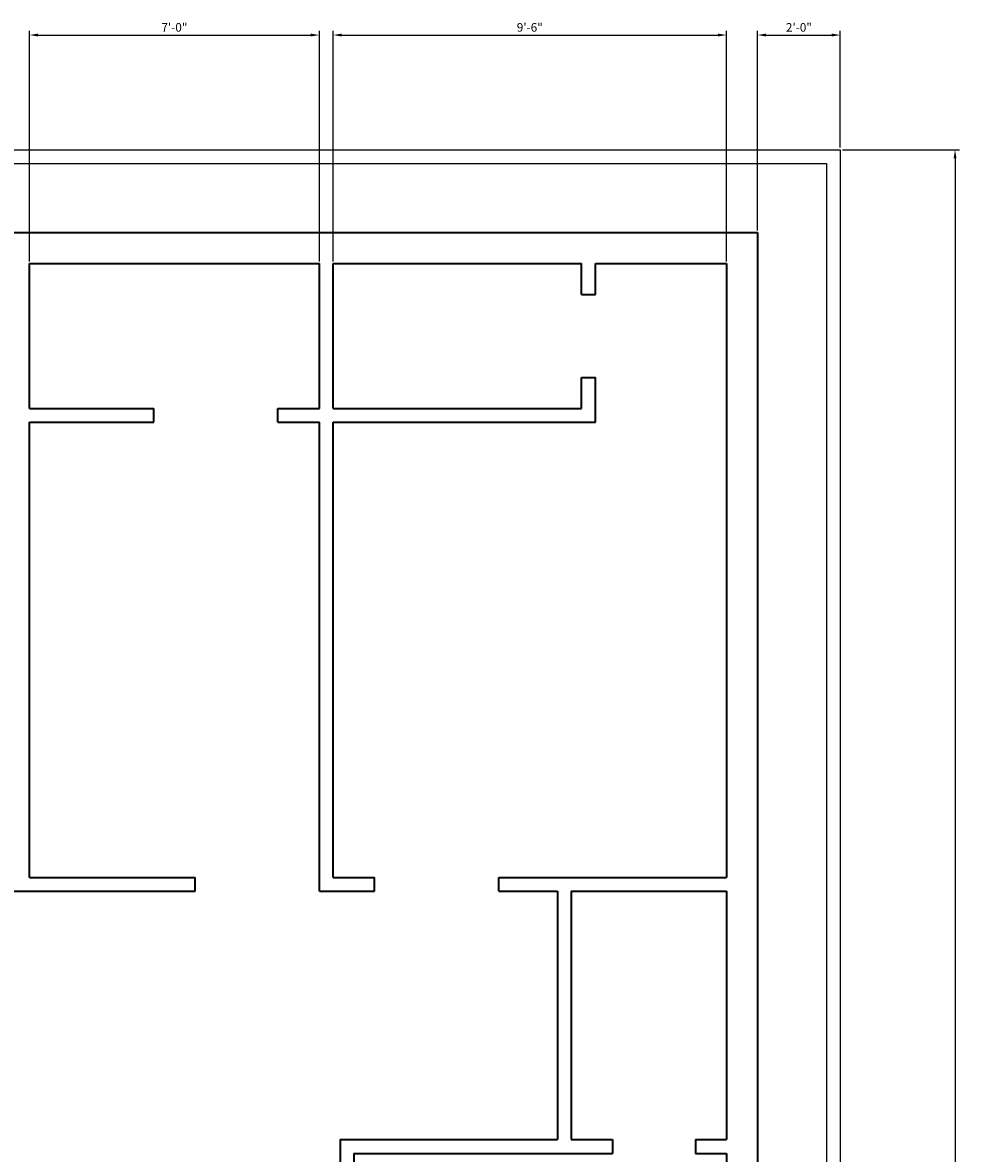
# Model space of a CAD drawing. Units: inches. Extents: x 2169 to 10664, y 1669 to 6352.
# Tile 12 of 17: x 4677 to 4948, y 2329 to 2657. Entities that reach past the tile are written whole.
import ezdxf

# ---------------------------------------------------------------- set-up
doc = ezdxf.new("R2010")
doc.units = ezdxf.units.IN
for name, color, linetype, lineweight in [('A-ANNO-DIMS', 3, 'Continuous', 18), ('A-WALL', 7, 'Continuous', 35), ('C-PROP', 251, 'Continuous', 25)]:
    doc.layers.add(name, color=color, linetype=linetype, lineweight=lineweight)
doc.styles.get("Standard").update_dxf_attribs({"font": 'arial.ttf'})
doc.dimstyles.new('ISO-25', dxfattribs={"dimtxt": 2.5, "dimasz": 2.5, "dimexe": 1.25, "dimexo": 0.625, "dimtad": 1, "dimdec": 0, "dimlunit": 3, "dimtxsty": 'Standard', "dimcen": 2.5, "dimadec": 0, "dimazin": 0, "dimtfac": 1, "dimtdec": 0, "dimtmove": 0, "dimatfit": 3, "dimfxl": 1, "dimarcsym": 0})

# ---------------------------------------------------------------- blocks, each defined once
blk = doc.blocks.new('*D103')
at = {"layer": 'A-ANNO-DIMS', "color": 0, "lineweight": -2, "transparency": 16777216}
for p, q in [((4914.2, 2620.19), (4948.07, 2620.19)), ((4946.82, 2617.69), (4946.82, 2004.69)), ((4914.2, 2002.19), (4948.07, 2002.19))]:
    blk.add_line(p, q, dxfattribs=at)
at = {"layer": 'A-ANNO-DIMS', "color": 0, "transparency": 16777216}
for points in [[(4946.41, 2617.69), (4947.24, 2617.69), (4946.82, 2620.19)], [(4946.41, 2004.69), (4947.24, 2004.69), (4946.82, 2002.19)]]:
    blk.add_solid(points, dxfattribs=at)
at = {"layer": 'Defpoints', "color": 0, "transparency": 16777216}
for p in [(4913.57, 2620.19), (4913.57, 2002.19), (4946.82, 2002.19)]:
    blk.add_point(p, dxfattribs=at)
at = {"layer": 'A-ANNO-DIMS', "color": 0, "transparency": 16777216, "insert": (4944.92, 2311.19), "char_height": 2.5, "attachment_point": 5, "rotation": 90}
blk.add_mtext('51\'-6"', dxfattribs=at)
blk = doc.blocks.new('*D107')
at = {"layer": 'A-ANNO-DIMS', "color": 0, "lineweight": -2, "transparency": 16777216}
for p, q in [((4678.57, 2587.81), (4678.57, 2654.69)), ((4681.07, 2653.44), (4760.07, 2653.44)), ((4762.57, 2587.81), (4762.57, 2654.69))]:
    blk.add_line(p, q, dxfattribs=at)
at = {"layer": 'A-ANNO-DIMS', "color": 0, "transparency": 16777216}
for points in [[(4681.07, 2653.86), (4681.07, 2653.02), (4678.57, 2653.44)], [(4760.07, 2653.86), (4760.07, 2653.02), (4762.57, 2653.44)]]:
    blk.add_solid(points, dxfattribs=at)
at = {"layer": 'Defpoints', "color": 0, "transparency": 16777216}
for p in [(4762.57, 2653.44), (4678.57, 2587.19), (4762.57, 2587.19)]:
    blk.add_point(p, dxfattribs=at)
at = {"layer": 'A-ANNO-DIMS', "color": 0, "transparency": 16777216, "insert": (4720.57, 2655.34), "char_height": 2.5, "attachment_point": 5}
blk.add_mtext('7\'-0"', dxfattribs=at)
blk = doc.blocks.new('*D108')
at = {"layer": 'A-ANNO-DIMS', "color": 0, "lineweight": -2, "transparency": 16777216}
for p, q in [((4766.57, 2587.81), (4766.57, 2654.69)), ((4769.07, 2653.44), (4878.07, 2653.44)), ((4880.57, 2587.81), (4880.57, 2654.69))]:
    blk.add_line(p, q, dxfattribs=at)
at = {"layer": 'A-ANNO-DIMS', "color": 0, "transparency": 16777216}
for points in [[(4769.07, 2653.86), (4769.07, 2653.02), (4766.57, 2653.44)], [(4878.07, 2653.86), (4878.07, 2653.02), (4880.57, 2653.44)]]:
    blk.add_solid(points, dxfattribs=at)
at = {"layer": 'Defpoints', "color": 0, "transparency": 16777216}
for p in [(4880.57, 2653.44), (4766.57, 2587.19), (4880.57, 2587.19)]:
    blk.add_point(p, dxfattribs=at)
at = {"layer": 'A-ANNO-DIMS', "color": 0, "transparency": 16777216, "insert": (4823.57, 2655.34), "char_height": 2.5, "attachment_point": 5}
blk.add_mtext('9\'-6"', dxfattribs=at)
blk = doc.blocks.new('*D109')
at = {"layer": 'A-ANNO-DIMS', "color": 0, "lineweight": -2, "transparency": 16777216}
for p, q in [((4889.57, 2596.81), (4889.57, 2654.69)), ((4892.07, 2653.44), (4911.07, 2653.44)), ((4913.57, 2620.81), (4913.57, 2654.69))]:
    blk.add_line(p, q, dxfattribs=at)
at = {"layer": 'A-ANNO-DIMS', "color": 0, "transparency": 16777216}
for points in [[(4892.07, 2653.86), (4892.07, 2653.02), (4889.57, 2653.44)], [(4911.07, 2653.86), (4911.07, 2653.02), (4913.57, 2653.44)]]:
    blk.add_solid(points, dxfattribs=at)
at = {"layer": 'Defpoints', "color": 0, "transparency": 16777216}
for p in [(4913.57, 2653.44), (4913.57, 2620.19), (4889.57, 2596.19)]:
    blk.add_point(p, dxfattribs=at)
at = {"layer": 'A-ANNO-DIMS', "color": 0, "transparency": 16777216, "insert": (4901.57, 2655.34), "char_height": 2.5, "attachment_point": 5}
blk.add_mtext('2\'-0"', dxfattribs=at)

msp = doc.modelspace()

# ---------------------------------------------------------------- linework, layer by layer
at = {"layer": 'A-WALL'}
for p, q in [((4457.57, 2596.19), (4889.57, 2596.19)), ((4889.57, 2596.19), (4889.57, 2080.19)), ((4678.57, 2587.19), (4762.57, 2587.19)), ((4678.57, 2545.19), (4678.57, 2587.19)), ((4762.57, 2545.19), (4762.57, 2587.19)), ((4766.57, 2587.19), (4838.57, 2587.19)), ((4766.57, 2545.19), (4766.57, 2587.19)), ((4838.57, 2578.19), (4838.57, 2587.19)), ((4842.57, 2578.19), (4842.57, 2587.19)), ((4842.57, 2587.19), (4880.57, 2587.19)), ((4880.57, 2587.19), (4880.57, 2409.19)), ((4838.57, 2578.19), (4842.57, 2578.19)), ((4838.57, 2545.19), (4838.57, 2554.19)), ((4838.57, 2554.19), (4842.57, 2554.19)), ((4842.57, 2541.19), (4842.57, 2554.19)), ((4678.57, 2545.19), (4714.57, 2545.19)), ((4714.57, 2541.19), (4714.57, 2545.19)), ((4750.57, 2541.19), (4750.57, 2545.19)), ((4750.57, 2545.19), (4762.57, 2545.19)), ((4766.57, 2545.19), (4838.57, 2545.19)), ((4678.57, 2409.19), (4678.57, 2541.19)), ((4678.57, 2541.19), (4714.57, 2541.19)), ((4750.57, 2541.19), (4762.57, 2541.19)), ((4762.57, 2405.19), (4762.57, 2541.19)), ((4766.57, 2409.19), (4766.57, 2541.19)), ((4766.57, 2541.19), (4842.57, 2541.19)), ((4678.57, 2409.19), (4726.57, 2409.19)), ((4726.57, 2405.19), (4726.57, 2409.19)), ((4766.57, 2409.19), (4778.57, 2409.19)), ((4778.57, 2405.19), (4778.57, 2409.19)), ((4814.57, 2405.19), (4814.57, 2409.19)), ((4814.57, 2409.19), (4880.57, 2409.19)), ((4642.57, 2405.19), (4726.57, 2405.19)), ((4762.57, 2405.19), (4778.57, 2405.19)), ((4814.57, 2405.19), (4831.57, 2405.19)), ((4831.57, 2405.19), (4831.57, 2333.19)), ((4835.57, 2405.19), (4835.57, 2333.19)), ((4835.57, 2405.19), (4880.57, 2405.19)), ((4880.57, 2405.19), (4880.57, 2333.19)), ((4768.57, 2333.19), (4831.57, 2333.19)), ((4768.57, 2333.19), (4768.57, 2237.19)), ((4835.57, 2333.19), (4847.57, 2333.19)), ((4847.57, 2333.19), (4847.57, 2329.19)), ((4871.57, 2333.19), (4871.57, 2329.19)), ((4871.57, 2333.19), (4880.57, 2333.19)), ((4772.57, 2329.19), (4847.57, 2329.19)), ((4772.57, 2329.19), (4772.57, 2237.19)), ((4871.57, 2329.19), (4880.57, 2329.19)), ((4880.57, 2329.19), (4880.57, 2189.19))]:
    msp.add_line(p, q, dxfattribs=at)
at = {"layer": 'C-PROP'}
for p, q in [((4433.57, 2620.19), (4913.57, 2620.19)), ((4913.57, 2620.19), (4913.57, 2002.19)), ((4437.57, 2616.19), (4909.57, 2616.19)), ((4909.57, 2616.19), (4909.57, 2002.19))]:
    msp.add_line(p, q, dxfattribs=at)

# ---------------------------------------------------------------- dimensions: what is measured, and where the dimension line sits
at = {"layer": 'A-ANNO-DIMS'}
for base, p1, p2, picture, middle in [((4762.57, 2653.44), (4678.57, 2587.19), (4762.57, 2587.19), '*D107', (4720.57, 2655.34)), ((4880.57, 2653.44), (4766.57, 2587.19), (4880.57, 2587.19), '*D108', (4823.57, 2655.34)), ((4913.57, 2653.44), (4889.57, 2596.19), (4913.57, 2620.19), '*D109', (4901.57, 2655.34))]:
    dim = msp.add_linear_dim(base=base, p1=p1, p2=p2, dimstyle='ISO-25', override={"dimdec": 1, "dimlfac": 1, "dimrnd": 0, "dimzin": 1, "dimdsep": 46, "dimlunit": 4, "dimfrac": 2}, dxfattribs=at)
    dim.commit()
    dim.dimension.update_dxf_attribs({"geometry": picture, "text_midpoint": middle})
dim = msp.add_linear_dim(base=(4946.82, 2002.19), p1=(4913.57, 2620.19), p2=(4913.57, 2002.19), angle=90, dimstyle='ISO-25', override={"dimdec": 1, "dimlfac": 1, "dimrnd": 0, "dimzin": 1, "dimdsep": 46, "dimlunit": 4, "dimfrac": 2}, dxfattribs=at)
dim.commit()
dim.dimension.update_dxf_attribs({"geometry": '*D103', "text_midpoint": (4944.92, 2311.19)})

doc.saveas('drawing.dxf')
